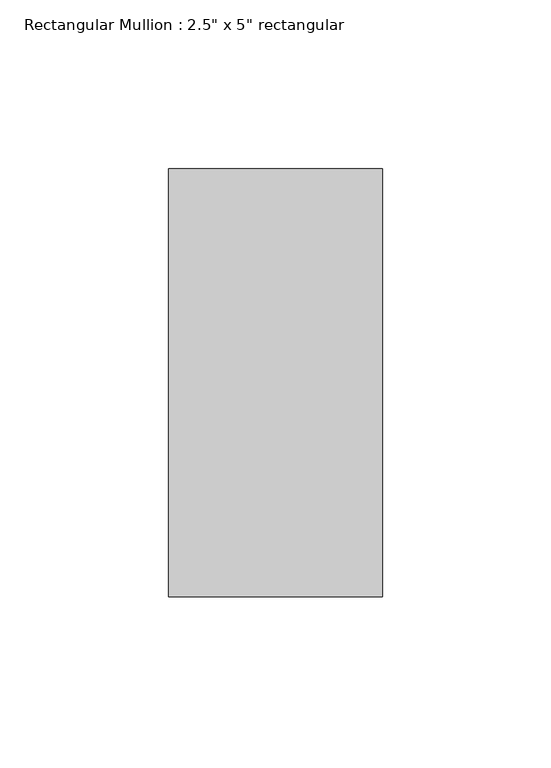
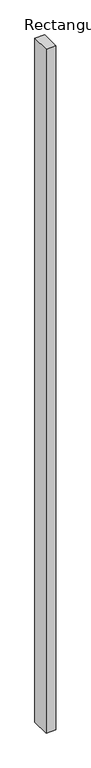
"""IFC4 building model written with IfcOpenShell, lengths in millimetres: member geometry."""

from ifc_helpers import new_model, si_unit, frame, origin, place, context, project, spatial, polyline, outline, extrude, source, transform, mapped, element, save


def member_23f0e500(model_context):
    return source(origin(), model_context, "Body", "SweptSolid", [
        extrude(outline(polyline([(0.0, 63.5), (0.0, -63.5), (-63.5, -63.5), (-63.5, 63.5), (0.0, 63.5)])), frame((0.0, 0.0, -4757.8664275), z_axis=(0.0, 0.0, 1.0), x_axis=(1.0, 0.0, 0.0)), (0.0, 0.0, 1.0), 4757.8664275),
    ])


if __name__ == "__main__":
    model = new_model("IFC4")
    model_context = context("Model", 3, world=origin())
    ifc_project = project(units=[si_unit("LENGTHUNIT", "METRE", prefix="MILLI")], contexts=[model_context])
    site = spatial("IfcSite", under=ifc_project)
    building = spatial("IfcBuilding", under=site)
    placement = place(None, origin())
    member_shape = member_23f0e500(model_context)
    element("IfcMember", 1, ObjectType="Rectangular Mullion : 2.5\" x 5\" rectangular", at=placement, inside=building, context=model_context, shape_type="MappedRepresentation", body=[
        mapped(member_shape, transform((0.0, 0.0, 0.0), x_axis=(1.0, 0.0, 0.0), y_axis=(0.0, 1.0, 0.0), z_axis=(0.0, 0.0, 1.0))),
    ])
    save(model, "model.ifc")

# Revit data of these elements
# Type "Rectangular Mullion : 2.5\" x 5\" rectangular"
#   built-in parameter 1007304 = 0.416667 (stored number, unit not read)
#   built-in parameter 1007301 = 0.104167 (stored number, unit not read)
#   built-in parameter 1007300 = 0.104167 (stored number, unit not read)
# Element 1 (IfcMember, "Rectangular Mullion : 2.5\" x 5\" rectangular")
#   Materials on its faces: "Aluminum"
# Materials
#   "Aluminum": class "Metal", colour RGB 247 247 247, transparency 0, Description = "Aluminum 6061", Cost = 0
